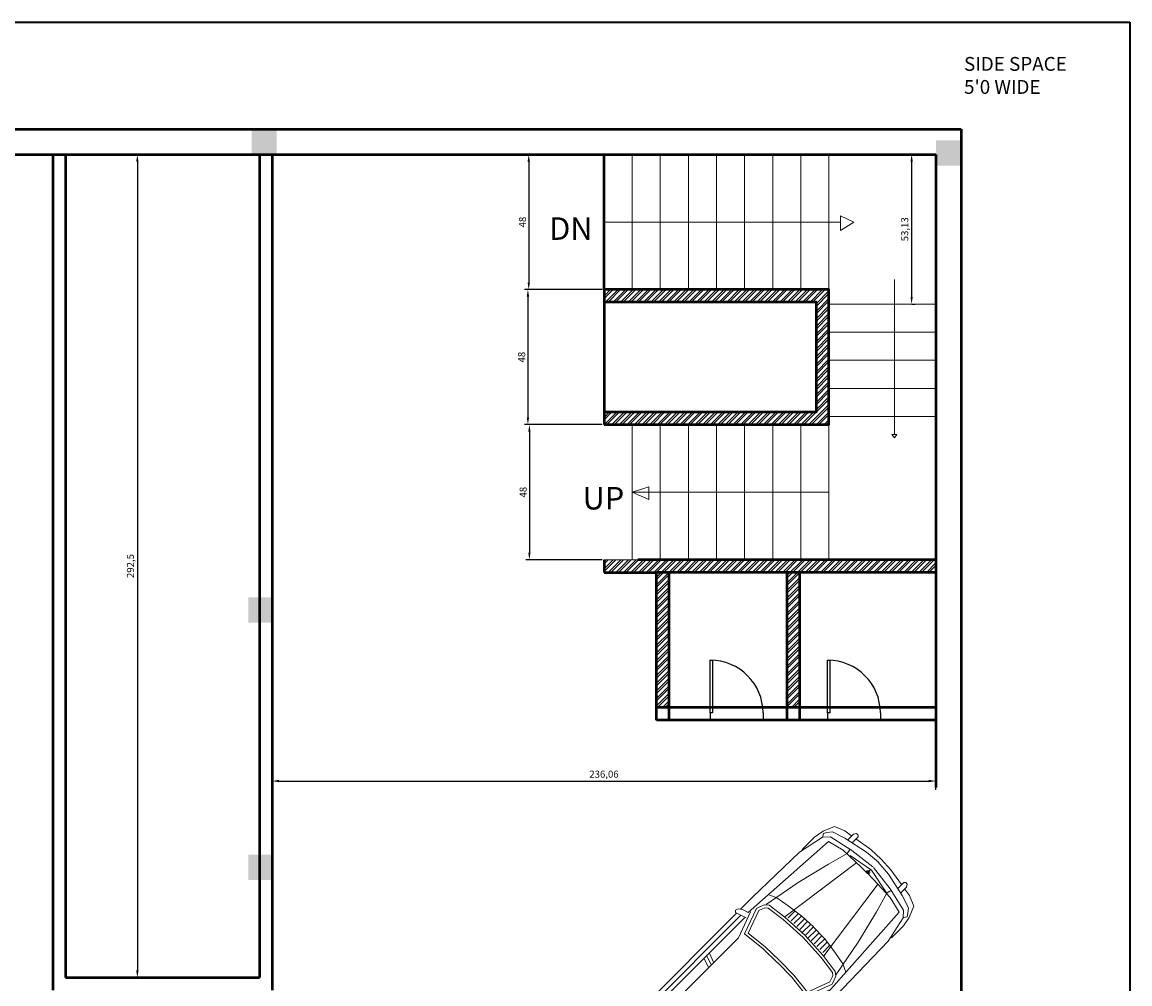
# Model space of a CAD drawing. Units: millimetres. Extents: x 2134 to 3363, y 1052 to 3233.
# Tile 9 of 11: x 2770 to 3164, y 2718 to 3059. Entities that reach past the tile are written whole.
import ezdxf

# ---------------------------------------------------------------- set-up
doc = ezdxf.new("R2010")
doc.units = ezdxf.units.MM
for name, color, linetype, lineweight in [('A-ANNO-DIMS', 2, 'Continuous', 18), ('A-ANNO-TEXT', 7, 'Continuous', 18), ('A-AREA-IDEN', 3, 'Continuous', 18), ('A-COLS', 1, 'Continuous', 35), ('A-DOOR', 4, 'Continuous', 25), ('A-FLOR-STRS', 3, 'Continuous', 18), ('A-SITE-PRKG', 8, 'Continuous', 13), ('A-WALL', 7, 'Continuous', 50), ('A-WALL-PATT', 8, 'Continuous', 13), ('C-PROP', 6, 'Continuous', 35)]:
    doc.layers.add(name, color=color, linetype=linetype, lineweight=lineweight)
doc.styles.get("Standard").update_dxf_attribs({"font": 'arial.ttf'})
doc.styles.add('YQ_DIM', font='SUPEROS.SHX', dxfattribs={"width": 0.8, "bigfont": 'HZDX.SHX'})
doc.dimstyles.new('ISO-25', dxfattribs={"dimtxt": 2.5, "dimasz": 2.5, "dimexe": 1.25, "dimexo": 0.625, "dimtad": 1, "dimtxsty": 'Standard', "dimcen": 2.5, "dimadec": 0, "dimazin": 0, "dimtfac": 1, "dimtmove": 0, "dimatfit": 3, "dimfxl": 1, "dimarcsym": 0})

# ---------------------------------------------------------------- blocks, each defined once
blk = doc.blocks.new('A$C49703025')
for p, q in [((2.816, 0.829), (2.838, 0.849)), ((2.838, 0.849), (2.874, 0.835)), ((-0.077, 0.686), (-0.044, 0.735)), ((-0.044, 0.735), (0.024, 0.765)), ((0.024, 0.765), (0.105, 0.775)), ((0.105, 0.735), (0.057, 0.691)), ((0.061, 0.671), (0.683, 0.735)), ((0.388, 0.78), (0.105, 0.735)), ((0.105, 0.775), (0.174, 0.75)), ((0.804, 0.813), (0.388, 0.78)), ((0.683, 0.735), (1.027, 0.755)), ((2.822, 0.813), (0.804, 0.813)), ((1.027, 0.755), (2.841, 0.755)), ((1.443, 0.586), (1.212, 0.702)), ((1.212, 0.702), (2.85, 0.702)), ((2.958, 0.702), (2.618, 0.575)), ((2.864, 0.684), (2.816, 0.829)), ((2.874, 0.835), (2.905, 0.791)), ((3.1, 0.813), (2.89, 0.813)), ((2.905, 0.791), (2.932, 0.714)), ((2.932, 0.714), (4.286, 0.632)), ((3.929, 0.795), (3.1, 0.813)), ((4.269, 0.722), (3.929, 0.795)), ((3.993, 0.795), (3.965, 0.787)), ((4.2, 0.795), (3.993, 0.795)), ((4.328, 0.77), (4.2, 0.795)), ((4.343, 0.656), (4.269, 0.722)), ((4.279, 0.724), (4.312, 0.747)), ((4.312, 0.747), (4.35, 0.724)), ((4.472, 0.711), (4.328, 0.77)), ((4.35, 0.724), (4.407, 0.681)), ((4.525, 0.578), (4.472, 0.711)), ((-0.093, 0.489), (-0.089, 0.573)), ((-0.089, 0.573), (-0.077, 0.686)), ((0.057, 0.691), (0.02, 0.543)), ((0.881, 0.661), (0.04, 0.607)), ((0.707, 0.469), (0.792, 0.652)), ((0.808, 0.597), (0.732, 0.444)), ((0.877, 0.652), (0.808, 0.597)), ((0.942, 0.661), (0.877, 0.652)), ((1.002, 0.652), (0.942, 0.661)), ((1.152, 0.617), (1.002, 0.652)), ((1.217, 0.573), (1.152, 0.617)), ((1.221, 0.528), (1.217, 0.573)), ((1.507, 0.575), (1.443, 0.586)), ((2.618, 0.575), (1.507, 0.575)), ((1.538, 0.592), (1.529, 0.68)), ((1.566, 0.592), (1.557, 0.68)), ((2.125, 0.696), (2.083, 0.58)), ((2.174, 0.695), (2.132, 0.579)), ((2.219, 0.697), (2.178, 0.581)), ((2.707, 0.554), (3.041, 0.676)), ((2.747, 0.529), (3.041, 0.637)), ((3.041, 0.676), (3.144, 0.639)), ((3.041, 0.637), (3.122, 0.608)), ((3.122, 0.608), (3.148, 0.576)), ((3.144, 0.639), (3.183, 0.591)), ((3.148, 0.576), (3.18, 0.34)), ((3.163, 0.627), (3.648, 0.536)), ((3.183, 0.591), (3.217, 0.343)), ((3.317, 0.591), (3.271, 0.695)), ((3.35, 0.417), (3.317, 0.591)), ((4.286, 0.632), (4.337, 0.422)), ((4.412, 0.343), (4.343, 0.656)), ((4.407, 0.681), (4.461, 0.513)), ((4.542, 0.474), (4.525, 0.578)), ((-0.113, 0.489), (-0.053, 0.489)), ((-0.113, 0.42), (-0.113, 0.489)), ((-0.053, 0.489), (-0.053, 0.42)), ((0.02, 0.543), (0, 0.222)), ((0.667, 0.336), (0.707, 0.469)), ((0.732, 0.444), (0.679, 0.193)), ((1.221, 0.4), (1.221, 0.528)), ((2.741, 0.254), (2.707, 0.554)), ((2.778, 0.256), (2.747, 0.529)), ((3.648, 0.536), (4.083, 0.427)), ((4.083, 0.427), (4.344, 0.354)), ((4.337, 0.422), (4.348, 0.111)), ((4.461, 0.513), (4.529, 0.197)), ((4.473, 0.474), (4.574, 0.474)), ((4.574, 0.474), (4.606, 0.455)), ((4.609, 0.429), (4.592, 0.408)), ((4.606, 0.455), (4.609, 0.429)), ((-0.053, 0.42), (-0.113, 0.42)), ((-0.101, 0.306), (-0.096, 0.42)), ((-0.101, 0), (-0.101, 0.306)), ((0.643, 0.173), (0.667, 0.336)), ((1.196, 0), (1.221, 0.4)), ((3.18, 0.34), (3.198, 0)), ((3.217, 0.343), (3.235, 0.002)), ((3.22, 0.35), (4.35, 0.19)), ((3.241, 0.309), (3.365, 0.309)), ((3.38, 0.202), (3.35, 0.417)), ((4.344, 0.354), (4.395, 0.364)), ((4.415, -0.011), (4.354, 0.313)), ((4.395, 0.364), (4.404, 0.379)), ((4.456, 0.006), (4.412, 0.343)), ((4.592, 0.408), (4.49, 0.408)), ((4.59, 0.18), (4.553, 0.408)), ((0, 0.222), (0, 0)), ((0.635, 0), (0.643, 0.173)), ((0.679, 0.193), (0.671, 0)), ((2.744, 0.002), (2.741, 0.254)), ((2.781, 0.003), (2.778, 0.256)), ((3.241, 0.257), (3.373, 0.257)), ((3.241, 0.206), (3.382, 0.206)), ((3.241, 0.154), (3.382, 0.154)), ((3.386, 0.002), (3.38, 0.202)), ((4.529, 0.197), (4.546, -0.002)), ((4.599, 0), (4.59, 0.18)), ((-0.101, 0), (-0.101, -0.306)), ((0, -0.222), (0, 0)), ((0.635, 0), (0.643, -0.173)), ((0.679, -0.193), (0.671, 0)), ((1.196, 0), (1.221, -0.4)), ((3.241, 0.103), (3.382, 0.103)), ((3.241, 0.051), (3.382, 0.051)), ((3.241, 0), (3.382, 0)), ((4.348, 0.111), (4.348, -0.004)), ((4.348, -0.111), (4.348, 0.004)), ((4.363, 0.028), (4.359, 0.005)), ((4.359, 0.005), (4.363, -0.023)), ((4.386, 0.005), (4.363, 0.028)), ((4.529, -0.197), (4.546, 0.002)), ((4.599, 0), (4.59, -0.18)), ((2.744, -0.002), (2.741, -0.254)), ((2.781, -0.003), (2.778, -0.256)), ((3.18, -0.34), (3.198, 0)), ((3.217, -0.343), (3.235, -0.002)), ((3.241, -0.051), (3.382, -0.051)), ((3.241, -0.103), (3.382, -0.103)), ((3.386, -0.002), (3.38, -0.202)), ((4.337, -0.422), (4.348, -0.111)), ((4.344, -0.347), (4.415, -0.011)), ((4.401, 0), (4.354, 0)), ((4.363, -0.023), (4.382, -0.011)), ((4.456, -0.006), (4.412, -0.343)), ((0.02, -0.543), (0, -0.222)), ((0.643, -0.173), (0.667, -0.336)), ((0.732, -0.444), (0.679, -0.193)), ((2.741, -0.254), (2.707, -0.554)), ((2.778, -0.256), (2.747, -0.529)), ((3.22, -0.35), (4.35, -0.19)), ((3.241, -0.154), (3.382, -0.154)), ((3.241, -0.206), (3.382, -0.206)), ((3.241, -0.257), (3.373, -0.257)), ((3.38, -0.202), (3.35, -0.417)), ((4.461, -0.513), (4.529, -0.197)), ((4.59, -0.18), (4.553, -0.408)), ((-0.053, -0.42), (-0.113, -0.42)), ((-0.113, -0.42), (-0.113, -0.489)), ((-0.101, -0.306), (-0.096, -0.42)), ((-0.053, -0.489), (-0.053, -0.42)), ((0.667, -0.336), (0.707, -0.469)), ((1.221, -0.4), (1.221, -0.528)), ((3.148, -0.576), (3.18, -0.34)), ((3.183, -0.591), (3.217, -0.343)), ((3.241, -0.309), (3.365, -0.309)), ((3.35, -0.417), (3.317, -0.591)), ((4.083, -0.427), (4.344, -0.354)), ((4.412, -0.343), (4.343, -0.656)), ((4.344, -0.354), (4.395, -0.364)), ((4.395, -0.364), (4.404, -0.379)), ((4.592, -0.408), (4.49, -0.408)), ((4.609, -0.429), (4.592, -0.408)), ((-0.113, -0.489), (-0.053, -0.489)), ((-0.093, -0.489), (-0.089, -0.573)), ((0.057, -0.691), (0.02, -0.543)), ((0.707, -0.469), (0.792, -0.652)), ((0.808, -0.597), (0.732, -0.444)), ((1.221, -0.528), (1.217, -0.573)), ((2.707, -0.554), (3.041, -0.676)), ((2.747, -0.529), (3.041, -0.637)), ((3.163, -0.627), (3.648, -0.536)), ((3.648, -0.536), (4.083, -0.427)), ((4.286, -0.632), (4.337, -0.422)), ((4.407, -0.681), (4.461, -0.513)), ((4.473, -0.474), (4.574, -0.474)), ((4.542, -0.474), (4.525, -0.578)), ((4.574, -0.474), (4.606, -0.455)), ((4.606, -0.455), (4.609, -0.429)), ((-0.089, -0.573), (-0.077, -0.686)), ((-0.077, -0.686), (-0.044, -0.735)), ((0.881, -0.661), (0.04, -0.607)), ((0.105, -0.735), (0.057, -0.691)), ((0.061, -0.671), (0.683, -0.735)), ((0.877, -0.652), (0.808, -0.597)), ((0.942, -0.661), (0.877, -0.652)), ((1.002, -0.652), (0.942, -0.661)), ((1.152, -0.617), (1.002, -0.652)), ((1.217, -0.573), (1.152, -0.617)), ((1.443, -0.586), (1.212, -0.702)), ((1.507, -0.575), (1.443, -0.586)), ((2.618, -0.575), (1.507, -0.575)), ((1.538, -0.592), (1.529, -0.68)), ((1.566, -0.592), (1.557, -0.68)), ((2.125, -0.696), (2.083, -0.58)), ((2.174, -0.695), (2.132, -0.579)), ((2.219, -0.697), (2.178, -0.581)), ((2.958, -0.702), (2.618, -0.575)), ((2.864, -0.684), (2.816, -0.829)), ((2.932, -0.714), (4.286, -0.632)), ((3.041, -0.637), (3.122, -0.608)), ((3.041, -0.676), (3.144, -0.639)), ((3.122, -0.608), (3.148, -0.576)), ((3.144, -0.639), (3.183, -0.591)), ((3.317, -0.591), (3.271, -0.695)), ((4.343, -0.656), (4.269, -0.722)), ((4.35, -0.724), (4.407, -0.681)), ((4.525, -0.578), (4.472, -0.711)), ((-0.044, -0.735), (0.024, -0.765)), ((0.024, -0.765), (0.105, -0.775)), ((0.388, -0.78), (0.105, -0.735)), ((0.105, -0.775), (0.174, -0.75)), ((0.804, -0.813), (0.388, -0.78)), ((0.683, -0.735), (1.027, -0.755)), ((2.822, -0.813), (0.804, -0.813)), ((1.027, -0.755), (2.841, -0.755)), ((1.212, -0.702), (2.85, -0.702)), ((2.816, -0.829), (2.838, -0.849)), ((2.838, -0.849), (2.874, -0.835)), ((2.874, -0.835), (2.905, -0.791)), ((3.1, -0.813), (2.89, -0.813)), ((2.905, -0.791), (2.932, -0.714)), ((3.929, -0.795), (3.1, -0.813)), ((4.269, -0.722), (3.929, -0.795)), ((3.993, -0.795), (3.965, -0.787)), ((4.2, -0.795), (3.993, -0.795)), ((4.328, -0.77), (4.2, -0.795)), ((4.279, -0.724), (4.312, -0.747)), ((4.312, -0.747), (4.35, -0.724)), ((4.472, -0.711), (4.328, -0.77))]:
    blk.add_line(p, q)
blk = doc.blocks.new('*D15')
at = {"layer": 'A-ANNO-DIMS', "color": 0, "lineweight": -2, "transparency": 16777216}
for p, q in [((2821.19, 3012.27), (2810.1, 3012.27)), ((2811.35, 3009.77), (2811.35, 2722.27)), ((2815.32, 2719.77), (2810.1, 2719.77))]:
    blk.add_line(p, q, dxfattribs=at)
at = {"layer": 'A-ANNO-DIMS', "color": 0, "transparency": 16777216}
for points in [[(2810.94, 3009.77), (2811.77, 3009.77), (2811.35, 3012.27)], [(2810.94, 2722.27), (2811.77, 2722.27), (2811.35, 2719.77)]]:
    blk.add_solid(points, dxfattribs=at)
at = {"layer": 'Defpoints', "color": 0, "transparency": 16777216}
for p in [(2821.81, 3012.27), (2811.35, 2719.77), (2815.94, 2719.77)]:
    blk.add_point(p, dxfattribs=at)
at = {"layer": 'A-ANNO-DIMS', "color": 0, "transparency": 16777216, "insert": (2809.22, 2866.02), "char_height": 2.5, "attachment_point": 5, "rotation": 90}
blk.add_mtext('292,5', dxfattribs=at)
blk = doc.blocks.new('*D17')
at = {"layer": 'A-ANNO-DIMS', "color": 0, "lineweight": -2, "transparency": 16777216}
for p, q in [((3084.45, 3012.27), (3087.98, 3012.27)), ((3086.73, 3009.77), (3086.73, 2961.65)), ((3086.81, 2959.15), (3087.98, 2959.15))]:
    blk.add_line(p, q, dxfattribs=at)
at = {"layer": 'A-ANNO-DIMS', "color": 0, "transparency": 16777216}
for points in [[(3086.32, 3009.77), (3087.15, 3009.77), (3086.73, 3012.27)], [(3086.32, 2961.65), (3087.15, 2961.65), (3086.73, 2959.15)]]:
    blk.add_solid(points, dxfattribs=at)
at = {"layer": 'Defpoints', "color": 0, "transparency": 16777216}
for p in [(3083.83, 3012.27), (3086.19, 2959.15), (3086.73, 2959.15)]:
    blk.add_point(p, dxfattribs=at)
at = {"layer": 'A-ANNO-DIMS', "color": 0, "transparency": 16777216, "insert": (3084.61, 2985.71), "char_height": 2.5, "attachment_point": 5, "rotation": 90}
blk.add_mtext('53,13', dxfattribs=at)
blk = doc.blocks.new('*D18')
at = {"layer": 'A-ANNO-DIMS', "color": 0, "lineweight": -2, "transparency": 16777216}
for p, q in [((2952.25, 3012.27), (2949.3, 3012.27)), ((2950.55, 3009.77), (2950.55, 2966.77)), ((2976.71, 2964.27), (2949.3, 2964.27))]:
    blk.add_line(p, q, dxfattribs=at)
at = {"layer": 'A-ANNO-DIMS', "color": 0, "transparency": 16777216}
for points in [[(2950.14, 3009.77), (2950.97, 3009.77), (2950.55, 3012.27)], [(2950.14, 2966.77), (2950.97, 2966.77), (2950.55, 2964.27)]]:
    blk.add_solid(points, dxfattribs=at)
at = {"layer": 'Defpoints', "color": 0, "transparency": 16777216}
for p in [(2952.88, 3012.27), (2950.55, 2964.27), (2977.34, 2964.27)]:
    blk.add_point(p, dxfattribs=at)
at = {"layer": 'A-ANNO-DIMS', "color": 0, "transparency": 16777216, "insert": (2948.65, 2988.27), "char_height": 2.5, "attachment_point": 5, "rotation": 90}
blk.add_mtext('48', dxfattribs=at)
blk = doc.blocks.new('*D19')
at = {"layer": 'A-ANNO-DIMS', "color": 0, "lineweight": -2, "transparency": 16777216}
for p, q in [((2976.71, 2964.27), (2949.01, 2964.27)), ((2950.26, 2961.77), (2950.26, 2918.77)), ((2976.71, 2916.27), (2949.01, 2916.27))]:
    blk.add_line(p, q, dxfattribs=at)
at = {"layer": 'A-ANNO-DIMS', "color": 0, "transparency": 16777216}
for points in [[(2949.85, 2961.77), (2950.68, 2961.77), (2950.26, 2964.27)], [(2949.85, 2918.77), (2950.68, 2918.77), (2950.26, 2916.27)]]:
    blk.add_solid(points, dxfattribs=at)
at = {"layer": 'Defpoints', "color": 0, "transparency": 16777216}
for p in [(2977.34, 2964.27), (2950.26, 2916.27), (2977.34, 2916.27)]:
    blk.add_point(p, dxfattribs=at)
at = {"layer": 'A-ANNO-DIMS', "color": 0, "transparency": 16777216, "insert": (2948.36, 2940.27), "char_height": 2.5, "attachment_point": 5, "rotation": 90}
blk.add_mtext('48', dxfattribs=at)
blk = doc.blocks.new('*D20')
at = {"layer": 'A-ANNO-DIMS', "color": 0, "lineweight": -2, "transparency": 16777216}
for p, q in [((2976.71, 2916.27), (2949.53, 2916.27)), ((2950.78, 2913.77), (2950.78, 2870.77)), ((2976.71, 2868.27), (2949.53, 2868.27))]:
    blk.add_line(p, q, dxfattribs=at)
at = {"layer": 'A-ANNO-DIMS', "color": 0, "transparency": 16777216}
for points in [[(2950.37, 2913.77), (2951.2, 2913.77), (2950.78, 2916.27)], [(2950.37, 2870.77), (2951.2, 2870.77), (2950.78, 2868.27)]]:
    blk.add_solid(points, dxfattribs=at)
at = {"layer": 'Defpoints', "color": 0, "transparency": 16777216}
for p in [(2977.34, 2916.27), (2950.78, 2868.27), (2977.34, 2868.27)]:
    blk.add_point(p, dxfattribs=at)
at = {"layer": 'A-ANNO-DIMS', "color": 0, "transparency": 16777216, "insert": (2948.88, 2892.27), "char_height": 2.5, "attachment_point": 5, "rotation": 90}
blk.add_mtext('48', dxfattribs=at)
blk = doc.blocks.new('*D21')
at = {"layer": 'A-ANNO-DIMS', "color": 0, "lineweight": -2, "transparency": 16777216}
for p, q in [((2859.28, 2786.48), (2859.28, 2790.85)), ((2861.78, 2789.6), (3092.84, 2789.6)), ((3095.34, 2786.48), (3095.34, 2790.85))]:
    blk.add_line(p, q, dxfattribs=at)
at = {"layer": 'A-ANNO-DIMS', "color": 0, "transparency": 16777216}
for points in [[(2861.78, 2790.01), (2861.78, 2789.18), (2859.28, 2789.6)], [(3092.84, 2790.01), (3092.84, 2789.18), (3095.34, 2789.6)]]:
    blk.add_solid(points, dxfattribs=at)
at = {"layer": 'Defpoints', "color": 0, "transparency": 16777216}
for p in [(3095.34, 2789.6), (2859.28, 2785.86), (3095.34, 2785.86)]:
    blk.add_point(p, dxfattribs=at)
at = {"layer": 'A-ANNO-DIMS', "color": 0, "transparency": 16777216, "insert": (2977.31, 2791.72), "char_height": 2.5, "width": 26.4154, "attachment_point": 5}
blk.add_mtext('236,06', dxfattribs=at)
blk = doc.blocks.new('*U5')
for p, q in [((0, 0), (0, -6)), ((40, 0), (40, -6))]:
    blk.add_line(p, q)
blk.add_lwpolyline([(0, 0), (0, 40), (1.75, 40), (1.75, 0)], close=True)
blk.add_arc((0, 0), 40, 0, 90)

msp = doc.modelspace()

# ---------------------------------------------------------------- hatches: boundary and pattern name
at = {"layer": 'A-COLS'}
h = msp.add_hatch(color=256, dxfattribs=at)
h.dxf.hatch_style = 1
h.paths.add_polyline_path([(2860.961, 3021.49), (2851.961, 3021.49), (2851.961, 3012.49), (2860.961, 3012.49)])
h = msp.add_hatch(color=256, dxfattribs=at)
h.dxf.hatch_style = 1
h.paths.add_polyline_path([(3104.339, 3017.375), (3095.339, 3017.375), (3095.339, 3008.375), (3104.339, 3008.375)])
h = msp.add_hatch(color=256, dxfattribs=at)
h.dxf.hatch_style = 1
h.paths.add_polyline_path([(2859.858, 2854.875), (2850.858, 2854.875), (2850.858, 2845.875), (2859.858, 2845.875)])
h = msp.add_hatch(color=256, dxfattribs=at)
h.dxf.hatch_style = 1
h.paths.add_polyline_path([(2859.858, 2763.375), (2850.858, 2763.375), (2850.858, 2754.375), (2859.858, 2754.375)])
at = {"layer": 'A-WALL-PATT'}
h = msp.add_hatch(dxfattribs=at)
h.set_pattern_fill('ANSI32', color=256, scale=0.2)
h.set_pattern_definition([(45, (2052.4981, 1503.6934), (-1.3470384, 1.3470384), []), (45, (2053.3961, 1503.6934), (-1.3470384, 1.3470384), [])])
h.paths.add_polyline_path([(3057.339, 2964.274), (2977.339, 2964.274), (2977.339, 2959.774), (3052.839, 2959.774), (3052.839, 2920.774), (2977.339, 2920.774), (2977.339, 2916.274), (3057.339, 2916.274)])
h.paths.add_polyline_path([(3095.339, 2868.274), (2989.339, 2868.274), (2977.339, 2868.274), (2977.339, 2863.774), (2995.997, 2863.774), (3095.339, 2863.774)])
h.paths.add_polyline_path([(3046.997, 2863.774), (3042.497, 2863.774), (3042.497, 2815.774), (3046.997, 2815.774)])
h.paths.add_polyline_path([(3000.497, 2863.774), (2995.997, 2863.774), (2995.997, 2815.774), (3000.497, 2815.774)])

# ---------------------------------------------------------------- linework, layer by layer
at = {"layer": 'A-FLOR-STRS'}
for p, q in [((2977.339, 3012.274), (2977.339, 2964.274)), ((2987.339, 3012.274), (2987.339, 2964.274)), ((2997.339, 3012.274), (2997.339, 2964.274)), ((3007.339, 3012.274), (3007.339, 2964.274)), ((3017.339, 3012.274), (3017.339, 2964.274)), ((3027.339, 3012.274), (3027.339, 2964.274)), ((3037.339, 3012.274), (3037.339, 2964.274)), ((3047.339, 3012.274), (3047.339, 2964.274)), ((3057.339, 3012.274), (3057.339, 2964.274)), ((2977.339, 2988.274), (3061.432, 2988.274)), ((3080.684, 2967.908), (3080.684, 2912.732)), ((3057.339, 2959.149), (3095.339, 2959.149)), ((3057.339, 2949.149), (3095.339, 2949.149)), ((3057.339, 2939.149), (3095.339, 2939.149)), ((3057.339, 2929.149), (3095.339, 2929.149)), ((2987.339, 2868.274), (2987.339, 2916.274)), ((2997.339, 2868.274), (2997.339, 2916.274)), ((3007.339, 2868.274), (3007.339, 2916.274)), ((3017.339, 2868.274), (3017.339, 2916.274)), ((3027.339, 2868.274), (3027.339, 2916.274)), ((3037.339, 2868.274), (3037.339, 2916.274)), ((3047.339, 2868.274), (3047.339, 2916.274)), ((3057.339, 2919.149), (3095.339, 2919.149)), ((3057.339, 2868.274), (3057.339, 2916.274)), ((3095.339, 2868.274), (3095.339, 2916.274)), ((3080.684, 2912.742), (3079.665, 2912.742)), ((3079.665, 2912.742), (3080.684, 2911.606)), ((3080.684, 2914.287), (3080.684, 2912.742)), ((3080.684, 2912.732), (3081.526, 2912.732)), ((3081.526, 2912.732), (3080.684, 2911.606)), ((2987.339, 2892.274), (3057.339, 2892.274)), ((2989.339, 2868.274), (2977.339, 2868.274))]:
    msp.add_line(p, q, dxfattribs=at)
for points in [[(3061.432, 2990.517), (3061.432, 2985.267), (3066.184, 2988.274)], [(2993.282, 2889.683), (2987.339, 2892.274), (2993.282, 2894.194)]]:
    msp.add_lwpolyline(points, close=True, dxfattribs=at)
at = {"layer": 'A-WALL'}
for p, q in [((2554.198, 3021.274), (3104.339, 3021.274)), ((2575.001, 3021.274), (3104.339, 3021.274)), ((3104.339, 3021.274), (3104.339, 2017.274)), ((3104.339, 3021.274), (3104.339, 2006.774)), ((2562.739, 3012.274), (3095.339, 3012.274)), ((2567.009, 3012.274), (3095.339, 3012.274)), ((2781.282, 3012.274), (2781.282, 2715.274)), ((2785.782, 3012.274), (2785.782, 2719.774)), ((2854.782, 3012.274), (2854.782, 2719.774)), ((2859.282, 3012.274), (2859.282, 2715.274)), ((2977.339, 2964.274), (2977.339, 3012.274)), ((3095.339, 3012.274), (3095.339, 2787.274)), ((2977.339, 2868.274), (2977.339, 2863.774)), ((3095.339, 2868.274), (2989.339, 2868.274)), ((2977.339, 2863.774), (2995.997, 2863.774)), ((3095.339, 2863.774), (2995.997, 2863.774)), ((2995.997, 2811.274), (2995.997, 2863.774)), ((3000.497, 2811.274), (3000.497, 2863.774)), ((3042.497, 2811.274), (3042.497, 2863.774)), ((3046.997, 2811.274), (3046.997, 2863.774)), ((3095.339, 2815.774), (2995.997, 2815.774)), ((3095.339, 2811.274), (2995.997, 2811.274)), ((2785.782, 2719.774), (2854.782, 2719.774))]:
    msp.add_line(p, q, dxfattribs=at)
msp.add_lwpolyline([(2977.339, 2916.274), (3057.339, 2916.274), (3057.339, 2964.274), (2977.339, 2964.274)], close=True, dxfattribs=at)
msp.add_lwpolyline([(2977.339, 2920.774), (3052.839, 2920.774), (3052.839, 2959.774), (2977.339, 2959.774)], dxfattribs=at)
at = {"layer": 'C-PROP'}
for p, q in [((2496.11, 3059.32), (3164.339, 3059.32)), ((3164.339, 3059.32), (3164.339, 1770.366))]:
    msp.add_line(p, q, dxfattribs=at)

# ---------------------------------------------------------------- block references
at = {"layer": 'A-DOOR', "xscale": 0.468784832216934, "yscale": 0.468784832216934, "zscale": 0.468784832216934}
for p in [(3015.132, 2813.793), (3056.863, 2813.793)]:
    msp.add_blockref('*U5', p, dxfattribs=at)
at = {"layer": 'A-SITE-PRKG', "xscale": 28.10227870703558, "yscale": 28.10227870703558, "zscale": 28.10227870703558, "rotation": 45}
msp.add_blockref('A$C49703025', (2984.561, 2670.442), dxfattribs=at)

# ---------------------------------------------------------------- texts
at = {"layer": 'A-ANNO-TEXT', "char_height": 8, "attachment_point": 1, "style": 'YQ_DIM'}
for s, insert in [('{\\fSitka Banner Semibold|b1|i0|c0|p2;DN}', (2957.841, 2989.95)), ('{\\fSitka Banner Semibold|b1|i0|c0|p2;UP}', (2969.718, 2894.114))]:
    msp.add_mtext_dynamic_manual_height_columns(s, width=3.68944, gutter_width=12.5, heights=[0], dxfattribs=dict(at, insert=insert))
at = {"layer": 'A-AREA-IDEN', "insert": (3105.367, 3046.941), "char_height": 4.91305, "attachment_point": 1, "style": 'YQ_DIM'}
msp.add_mtext_dynamic_manual_height_columns("{\\f@Arial Unicode MS|b0|i0|c134|p34;SIDE SPACE\\P5'0 WIDE}", width=92.43125, gutter_width=24.565, heights=[0], dxfattribs=at)

# ---------------------------------------------------------------- dimensions: what is measured, and where the dimension line sits
at = {"layer": 'A-ANNO-DIMS'}
for base, p1, p2, picture, middle in [((2811.352, 2719.774), (2821.814, 3012.274), (2815.945, 2719.774), '*D15', (2809.224, 2866.024)), ((2950.553, 2964.274), (2952.878, 3012.274), (2977.339, 2964.274), '*D18', (2948.651, 2988.274)), ((3086.7332, 2959.1485), (3083.8292, 3012.2736), (3086.1887, 2959.1485), '*D17', (3084.6058, 2985.711)), ((2950.262, 2916.274), (2977.339, 2964.274), (2977.339, 2916.274), '*D19', (2948.36, 2940.274)), ((2950.784, 2868.274), (2977.339, 2916.274), (2977.339, 2868.274), '*D20', (2948.882, 2892.274))]:
    dim = msp.add_linear_dim(base=base, p1=p1, p2=p2, angle=90, dimstyle='ISO-25', override={"dimclrd": 0, "dimclre": 0, "dimclrt": 0}, dxfattribs=at)
    dim.commit()
    dim.dimension.update_dxf_attribs({"geometry": picture, "text_midpoint": middle})
dim = msp.add_linear_dim(base=(3095.339, 2789.595), p1=(2859.282, 2785.856), p2=(3095.339, 2785.856), dimstyle='ISO-25', override={"dimclrd": 0, "dimclre": 0, "dimclrt": 0}, dxfattribs=at)
dim.commit()
dim.dimension.update_dxf_attribs({"geometry": '*D21', "text_midpoint": (2977.311, 2791.723)})

doc.saveas('drawing.dxf')
